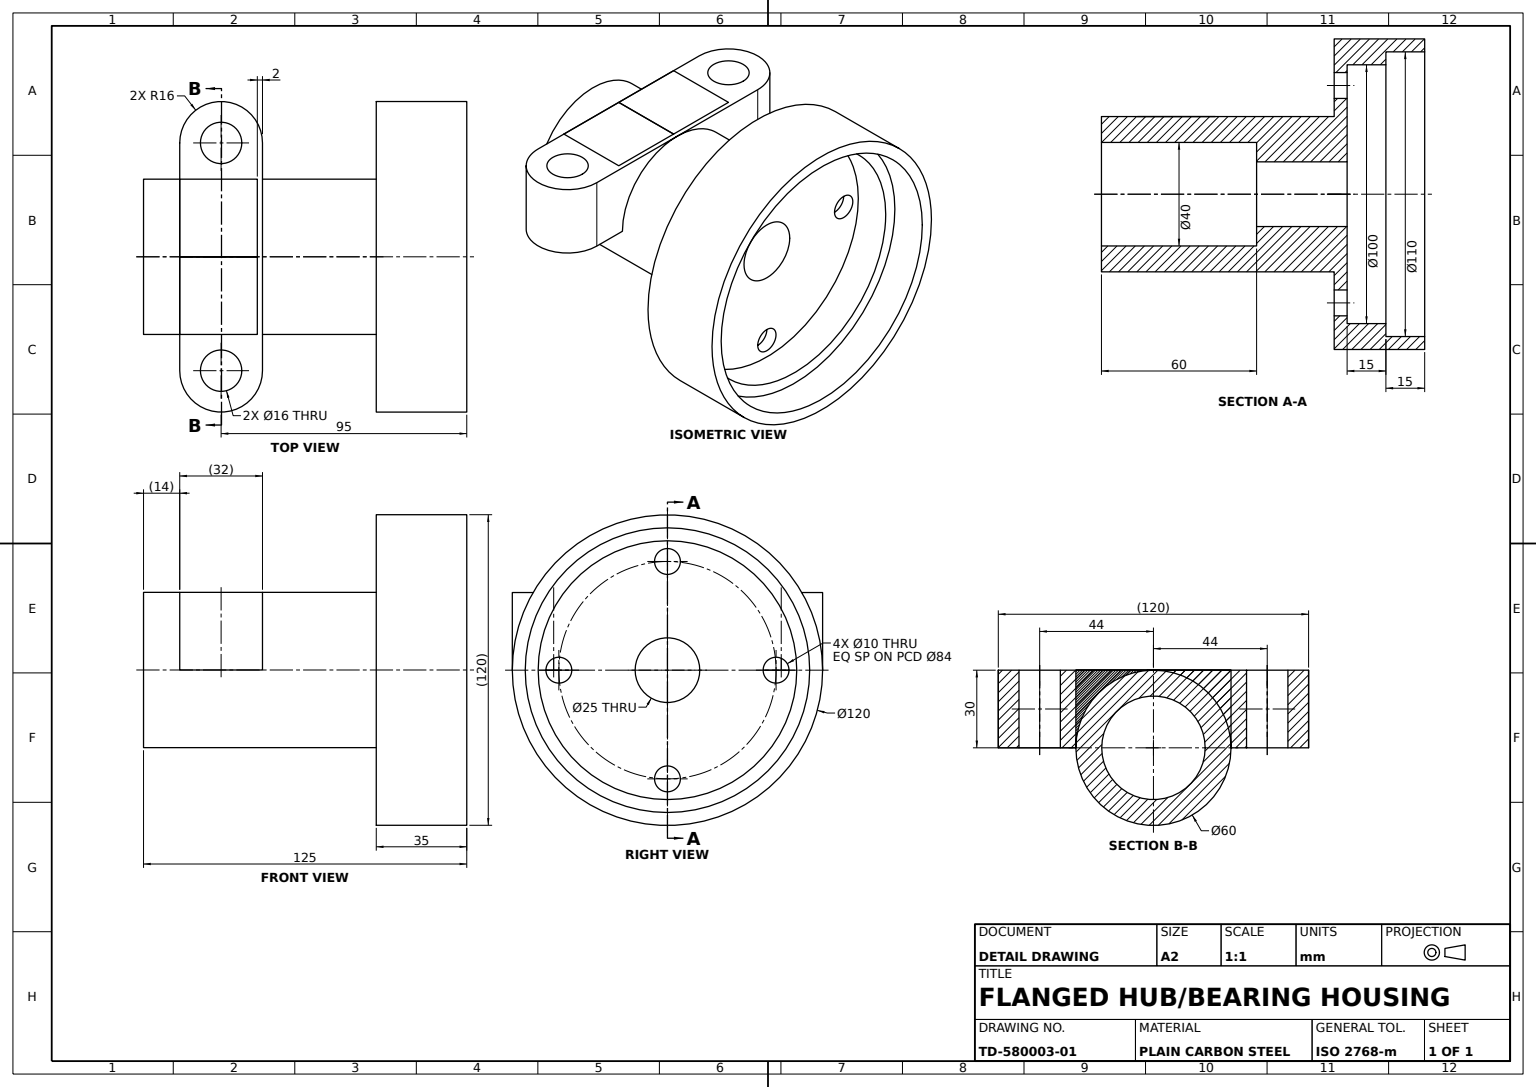
from build123d import *

# Parameters (mm, degrees)
FLANGE_SKETCH_120_R        = 60
FLANGE_120_DEPTH           = 35
FLANGE_RECESS_SKETCH_110_R = 55
FLANGE_RECESS_110_DEPTH    = 15
FLANGE_INNER_CUT_SKETCH_R  = 50
FLANGE_INNER_CUT_DEPTH     = 15
BOLT_HOLES_SKETCH_4X_10_R  = 5
BOLT_HOLES_4X_10_DEPTH     = 15
HUB_SKETCH_60_R            = 30
HUB_60_DEPTH               = 30
HUB_EXTENSION_DEPTH        = 60
CLAMP_LUGS_SKETCH_R        = 8
CLAMP_LUGS_DEPTH           = 30
CLAMP_LUGS_2_DEPTH         = 30
SHAFT_BORE_SKETCH_R        = 12.5
SHAFT_BORE_DEPTH           = 113
HUB_START                  = -60
HUB_TUBE_SKETCH_60_40_R    = 30
HUB_TUBE_SKETCH_60_40_R_2  = 20
HUB_TUBE_DEPTH             = 60
LUG_START                  = -32
LUG_WEB_B_DEPTH            = 32
LUG_WEB_A_DEPTH            = 30
LUG_WEB_A_2_DEPTH          = 30


with BuildPart() as part:
    # Flange Sketch Ø120 → Flange Ø120 (new body)
    with BuildSketch(Plane.XY):
        Circle(FLANGE_SKETCH_120_R)
    extrude(amount=FLANGE_120_DEPTH)

    # Flange Recess Sketch Ø110 → Flange Recess Ø110 (cut)
    with BuildSketch(Plane(origin=(0, 0, 0), x_dir=(-1, 0, 0), z_dir=(0, 0, -1))):
        Circle(FLANGE_RECESS_SKETCH_110_R)
    extrude(amount=-FLANGE_RECESS_110_DEPTH, mode=Mode.SUBTRACT)

    # Flange Inner Cut Sketch → Flange Inner Cut (cut)
    with BuildSketch(Plane(origin=(0, 0, 15), x_dir=(-1, 0, 0), z_dir=(0, 0, -1))):
        Circle(FLANGE_INNER_CUT_SKETCH_R)
    extrude(amount=-FLANGE_INNER_CUT_DEPTH, mode=Mode.SUBTRACT)

    # Bolt Holes Sketch 4xØ10 → Bolt Holes 4xØ10 (cut)
    with BuildSketch(Plane.XY.offset(35)):
        with Locations((42, 0)):
            Circle(BOLT_HOLES_SKETCH_4X_10_R)
        with Locations((0, -42)):
            Circle(BOLT_HOLES_SKETCH_4X_10_R)
        with Locations((-42, 0)):
            Circle(BOLT_HOLES_SKETCH_4X_10_R)
        with Locations((0, 42)):
            Circle(BOLT_HOLES_SKETCH_4X_10_R)
    extrude(amount=-BOLT_HOLES_4X_10_DEPTH, mode=Mode.SUBTRACT)

    # Hub Sketch Ø60 → Hub Ø60 (add)
    with BuildSketch(Plane.XY.offset(35)):
        Circle(HUB_SKETCH_60_R)
    extrude(amount=HUB_60_DEPTH)

    # Hub Extension Sketch → Hub Extension (add)
    with BuildSketch(Plane.XY.offset(65)):
        with BuildLine():
            Line((-30, 0), (-20, 0))
            ThreePointArc((-20, 0), (0, -20), (20, 0))
            Line((20, 0), (30, 0))
            ThreePointArc((30, 0), (0, -30), (-30, 0))
        make_face()
    extrude(amount=HUB_EXTENSION_DEPTH)

    # Shaft Bore Sketch → Shaft Bore (cut)
    with BuildSketch(Plane.XY.offset(65)):
        Circle(SHAFT_BORE_SKETCH_R)
    extrude(amount=-SHAFT_BORE_DEPTH, mode=Mode.SUBTRACT)

    # Hub Tube Sketch Ø60-Ø40 → Hub Tube (add)
    with BuildSketch(Plane.XY.offset(125).offset(HUB_START)):
        Circle(HUB_TUBE_SKETCH_60_40_R)
        with Locations(Location((0, 0, 0), (0, 0, 180))):
            Circle(HUB_TUBE_SKETCH_60_40_R_2, mode=Mode.SUBTRACT)
    extrude(amount=HUB_TUBE_DEPTH)



with BuildPart() as body_2:
    # Clamp Lugs Sketch → Clamp Lugs (new body)
    with BuildSketch(Plane(origin=(0, 0, 0), x_dir=(1, 0, 0), z_dir=(0, 1, 0))):
        with BuildLine():
            Line((44, -79), (30, -79))
            Line((30, -79), (30, -111))
            Line((30, -111), (44, -111))
            ThreePointArc((44, -111), (60, -95), (44, -79))
        make_face()
        with Locations(Location((44, -95, 0), (0, 0, 270))):
            Circle(CLAMP_LUGS_SKETCH_R, mode=Mode.SUBTRACT)
    extrude(amount=-CLAMP_LUGS_DEPTH)


with BuildPart() as body_3:
    # Clamp Lugs Sketch → Clamp Lugs 2 (new body)
    with BuildSketch(Plane(origin=(0, 0, 0), x_dir=(1, 0, 0), z_dir=(0, 1, 0))):
        with BuildLine():
            Line((-30, -111), (-44, -111))
            ThreePointArc((-44, -111), (-60, -95), (-44, -79))
            Line((-44, -79), (-30, -79))
            Line((-30, -79), (-30, -111))
        make_face()
        with Locations(Location((-44, -95, 0), (0, 0, 90))):
            Circle(CLAMP_LUGS_SKETCH_R, mode=Mode.SUBTRACT)
    extrude(amount=-CLAMP_LUGS_2_DEPTH)


with BuildPart() as part_1:
    add(part.part)

    add(body_2.part)  # Lug Web B merges body 2

    add(body_3.part)  # Lug Web B merges body 3
    # Lug Web B Sketch → Lug Web B (add)
    with BuildSketch(Plane.XY.offset(111).offset(LUG_START)):
        with BuildLine():
            Line((30, -30), (30, 0))
            ThreePointArc((30, 0), (21.213203436, -21.213203436), (0, -30))
            Line((0, -30), (30, -30))
        make_face()
        with BuildLine():
            Line((-30, -30), (0, -30))
            ThreePointArc((0, -30), (-21.213203436, -21.213203436), (-30, 0))
            Line((-30, 0), (-30, -30))
        make_face()
    extrude(amount=LUG_WEB_B_DEPTH)


with BuildPart() as body_2_2:
    # Lug Web A Sketch → Lug Web A (new body)
    with BuildSketch(Plane.XY.offset(111)):
        with BuildLine():
            Line((0, -30), (30, -30))
            Line((30, -30), (30, 0))
            ThreePointArc((30, 0), (21.213203436, -21.213203436), (0, -30))
        make_face()
    extrude(amount=-LUG_WEB_A_DEPTH)


with BuildPart() as body_3_2:
    # Lug Web A Sketch → Lug Web A 2 (new body)
    with BuildSketch(Plane.XY.offset(111)):
        with BuildLine():
            Line((-30, -30), (0, -30))
            ThreePointArc((0, -30), (-21.213203436, -21.213203436), (-30, 0))
            Line((-30, 0), (-30, -30))
        make_face()
    extrude(amount=-LUG_WEB_A_2_DEPTH)


solid = Compound([part_1.part, body_2_2.part, body_3_2.part])
